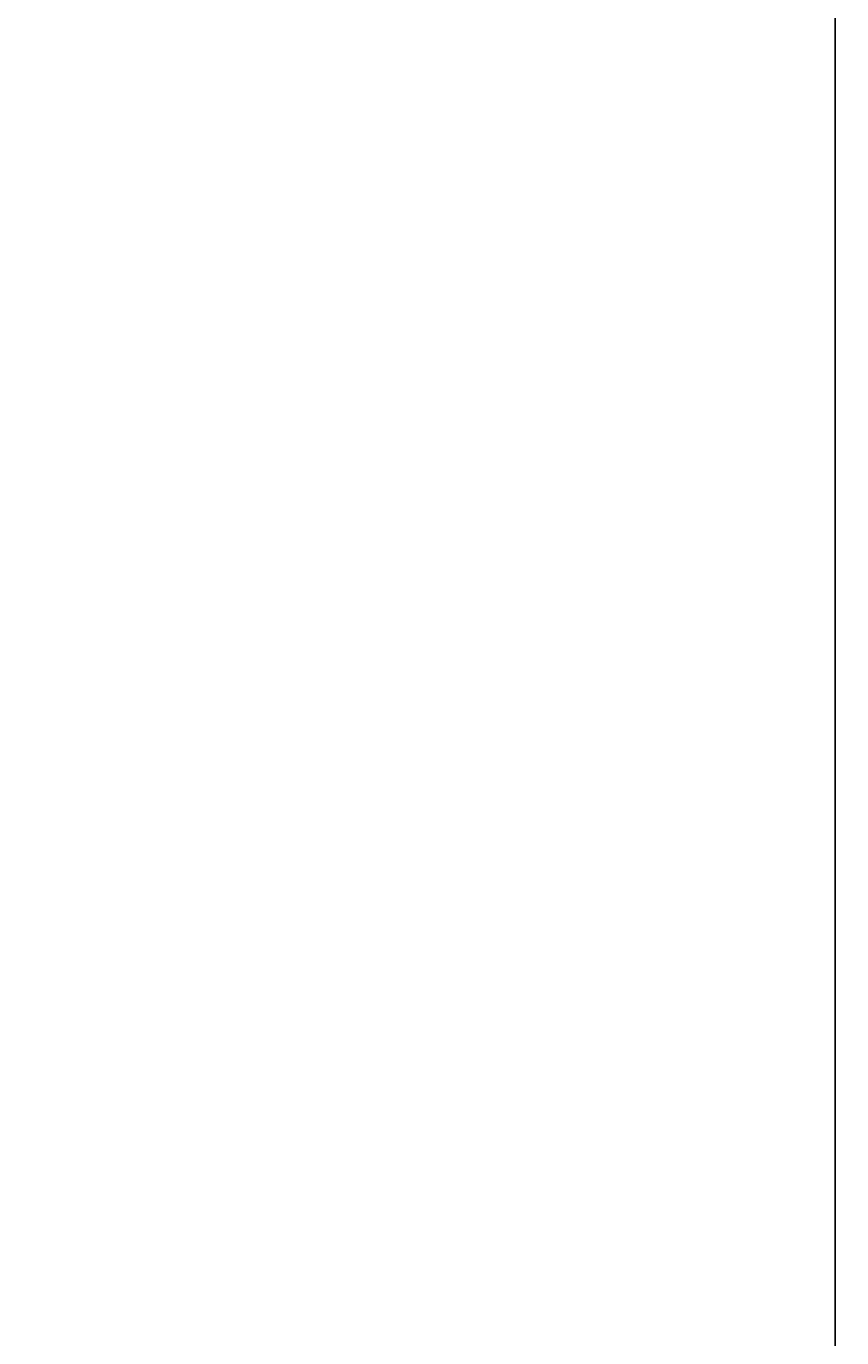
# Model space of a CAD drawing. Units: inches. Extents: x 1998 to 2588, y 1139 to 1977.
# Tile 132 of 134: x 2550 to 2588, y 1637 to 1698. Entities that reach past the tile are written whole.
import ezdxf

# ---------------------------------------------------------------- set-up
doc = ezdxf.new("R2010")
doc.units = ezdxf.units.IN
doc.layers.add('A-ANNO-DIMS', color=2, linetype='Continuous', lineweight=18)
doc.styles.get("Standard").update_dxf_attribs({"font": 'arial.ttf'})
doc.dimstyles.get("Standard").update_dxf_attribs({"dimtxt": 0.18, "dimasz": 0.18, "dimexe": 0.18, "dimexo": 0.0625, "dimgap": 0.09, "dimtad": 0, "dimtih": 1, "dimtoh": 1, "dimdec": 4, "dimzin": 0, "dimdsep": 46, "dimtxsty": 'Standard', "dimcen": 0.09, "dimadec": 0, "dimazin": 0, "dimtfac": 1, "dimtdec": 4, "dimtofl": 0, "dimtmove": 0, "dimatfit": 3, "dimfxl": 1, "dimtolj": 1, "dimtzin": 0, "dimarcsym": 0})

# ---------------------------------------------------------------- blocks, each defined once
blk = doc.blocks.new('*D24')
at = {"layer": 'A-ANNO-DIMS', "color": 0, "lineweight": -2, "transparency": 16777216}
for p, q in [((2398.535, 1911.232), (2588.309, 1911.232)), ((2588.129, 1911.052), (2588.129, 1570.164)), ((2588.129, 1228.912), (2588.129, 1569.8)), ((2527.535, 1228.732), (2588.309, 1228.732))]:
    blk.add_line(p, q, dxfattribs=at)
at = {"layer": 'A-ANNO-DIMS', "color": 0, "transparency": 16777216}
for points in [[(2588.099, 1911.052), (2588.159, 1911.052), (2588.129, 1911.232)], [(2588.099, 1228.912), (2588.159, 1228.912), (2588.129, 1228.732)]]:
    blk.add_solid(points, dxfattribs=at)
at = {"layer": 'Defpoints', "color": 0, "transparency": 16777216}
for p in [(2398.473, 1911.232), (2588.129, 1911.232), (2527.473, 1228.732)]:
    blk.add_point(p, dxfattribs=at)
at = {"layer": 'A-ANNO-DIMS', "color": 0, "transparency": 16777216, "insert": (2588.129, 1569.982), "char_height": 0.18, "attachment_point": 5}
blk.add_mtext('\\A1;682.5', dxfattribs=at)

msp = doc.modelspace()

# ---------------------------------------------------------------- dimensions: what is measured, and where the dimension line sits
at = {"layer": 'A-ANNO-DIMS'}
dim = msp.add_linear_dim(base=(2588.1286, 1911.2324), p1=(2527.4729, 1228.7324), p2=(2398.4729, 1911.2324), angle=90, dimstyle='Standard', override={"dimdec": 1, "dimlfac": 1, "dimrnd": 0, "dimzin": 0, "dimdsep": 46, "dimlunit": 2}, dxfattribs=at)
dim.commit()
dim.dimension.update_dxf_attribs({"geometry": '*D24', "text_midpoint": (2588.1286, 1569.9824)})

doc.saveas('drawing.dxf')
